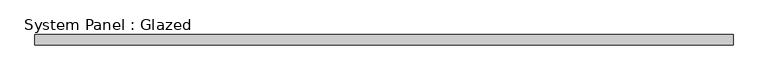
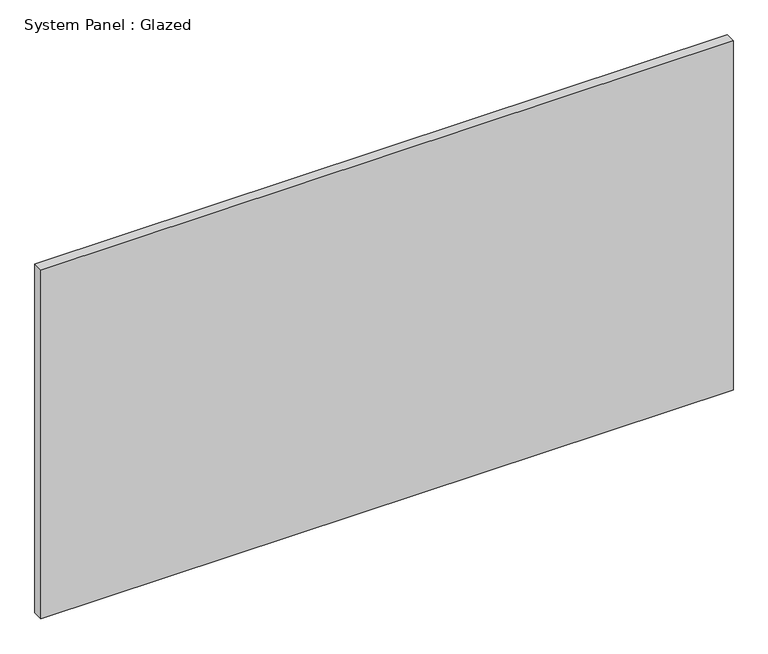
"""IFC4 building model written with IfcOpenShell, lengths in millimetres: plate geometry, System Panel : Glazed."""

from ifc_helpers import new_model, si_unit, origin, origin_with_axes, place, context, project, spatial, polyline, outline, extrude, source, transform, mapped, element, save


def system_panel_glazed_8f95e3f6(model_context):
    return source(origin(), model_context, "Body", "SweptSolid", [
        extrude(outline(polyline([(857.25, 19.05), (-857.25, 19.05), (-857.25, 44.45), (857.25, 44.45), (857.25, 19.05)])), origin_with_axes(), (0.0, 0.0, 1.0), 914.4),
    ])


if __name__ == "__main__":
    model = new_model("IFC4")
    model_context = context("Model", 3, world=origin())
    ifc_project = project(units=[si_unit("LENGTHUNIT", "METRE", prefix="MILLI")], contexts=[model_context])
    site = spatial("IfcSite", under=ifc_project)
    building = spatial("IfcBuilding", under=site)
    placement = place(None, origin())
    system_panel_glazed_shape = system_panel_glazed_8f95e3f6(model_context)
    element("IfcPlate", 1, ObjectType="System Panel : Glazed", at=placement, inside=building, context=model_context, shape_type="MappedRepresentation", body=[
        mapped(system_panel_glazed_shape, transform((0.0, 0.0, 0.0), x_axis=(1.0, 0.0, 0.0), y_axis=(0.0, 1.0, 0.0), z_axis=(0.0, 0.0, 1.0))),
    ])
    save(model, "model.ifc")

# Revit data of these elements
# Type "System Panel : Glazed"
#   Construction Type Id = "GSP4R"
#   Analytic Construction = "1/8 in Pilkington single glazing"
#   Visual Light Transmittance = 0.9
#   Solar Heat Gain Coefficient = 0.86
#   Heat Transfer Coefficient (U) = 6.7069 W/(m²·K)
# Element 1 (IfcPlate, "System Panel : Glazed")
#   Materials on its faces: "Glass"
# Materials
#   "Glass": class "Glass", colour RGB 0 128 192, transparency 0.75, Description = "Soda Lime Glass", Cost = 0
